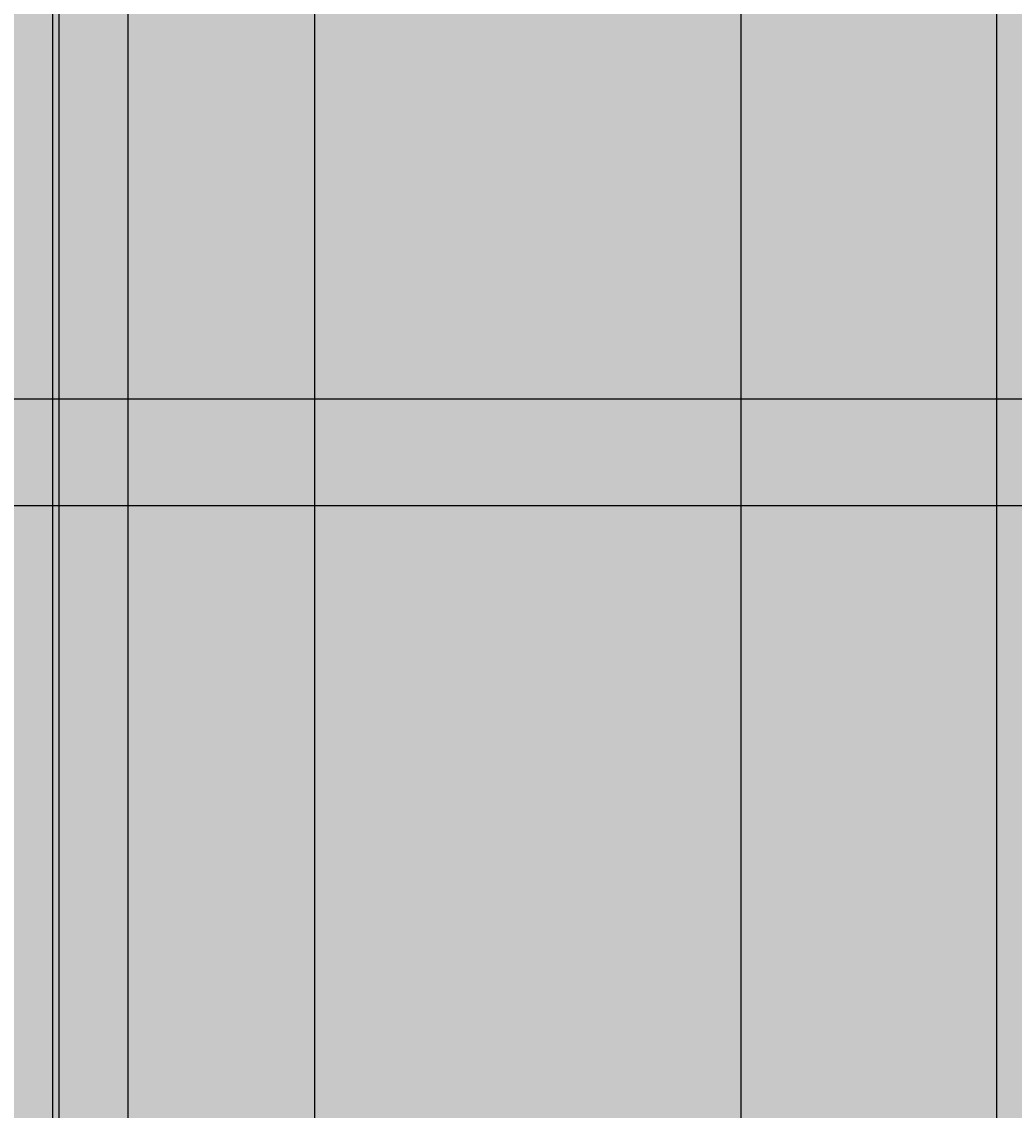
# Model space of a CAD drawing. Units: inches. Extents: x -12 to 334, y -10 to 186.
# Tile 64 of 77: x 216 to 239, y 111 to 137. Entities that reach past the tile are written whole.
import ezdxf

# ---------------------------------------------------------------- set-up
doc = ezdxf.new("R2010")
doc.units = ezdxf.units.IN
doc.header["$MEASUREMENT"] = 0
doc.layers.add('M-DIMS', color=2, linetype='Continuous', lineweight=18)
doc.layers.add('M-EQPM-PATT', color=8, linetype='Continuous', lineweight=18)
doc.styles.get("Standard").update_dxf_attribs({"font": 'arial.ttf'})
doc.dimstyles.get("Standard").update_dxf_attribs({"dimtxt": 0.18, "dimasz": 0.18, "dimexe": 0.18, "dimexo": 0.0625, "dimgap": 0.09, "dimtad": 0, "dimtih": 1, "dimtoh": 1, "dimdec": 4, "dimzin": 0, "dimdsep": 46, "dimtxsty": 'Standard', "dimcen": 0.09, "dimadec": 0, "dimazin": 0, "dimtfac": 1, "dimtdec": 4, "dimtofl": 0, "dimtmove": 0, "dimatfit": 3, "dimfxl": 1, "dimtolj": 1, "dimtzin": 0, "dimarcsym": 0})

# ---------------------------------------------------------------- blocks, each defined once
blk = doc.blocks.new('*D5')
at = {"layer": 'Defpoints', "color": 0, "transparency": 16777216}
for p in [(58.1, 127.708), (58.1, 125.208), (295.976, 125.208)]:
    blk.add_point(p, dxfattribs=at)
at = {"layer": 'M-DIMS', "color": 0, "lineweight": -2, "transparency": 16777216}
for p, q in [((58.163, 127.708), (296.156, 127.708)), ((295.976, 127.528), (295.976, 126.64)), ((295.976, 125.388), (295.976, 126.276)), ((58.163, 125.208), (296.156, 125.208))]:
    blk.add_line(p, q, dxfattribs=at)
at = {"layer": 'M-DIMS', "color": 0, "transparency": 16777216}
for points in [[(295.946, 127.528), (296.006, 127.528), (295.976, 127.708)], [(295.946, 125.388), (296.006, 125.388), (295.976, 125.208)]]:
    blk.add_solid(points, dxfattribs=at)
at = {"layer": 'M-DIMS', "color": 0, "transparency": 16777216, "insert": (295.976, 126.458), "char_height": 0.18, "attachment_point": 5}
blk.add_mtext('\\A1;2.5', dxfattribs=at)
blk = doc.blocks.new('*D27')
at = {"layer": 'Defpoints', "color": 0, "transparency": 16777216}
for p in [(238.576, 169.385), (216.576, 32.854), (238.576, 32.854)]:
    blk.add_point(p, dxfattribs=at)
at = {"layer": 'M-DIMS', "color": 0, "lineweight": -2, "transparency": 16777216}
for p, q in [((216.576, 32.917), (216.576, 169.565)), ((238.576, 32.917), (238.576, 169.565)), ((216.756, 169.385), (227.357, 169.385)), ((238.396, 169.385), (227.796, 169.385))]:
    blk.add_line(p, q, dxfattribs=at)
at = {"layer": 'M-DIMS', "color": 0, "transparency": 16777216}
for points in [[(216.756, 169.415), (216.756, 169.355), (216.576, 169.385)], [(238.396, 169.415), (238.396, 169.355), (238.576, 169.385)]]:
    blk.add_solid(points, dxfattribs=at)
at = {"layer": 'M-DIMS', "color": 0, "transparency": 16777216, "insert": (227.576, 169.385), "char_height": 0.18, "attachment_point": 5}
blk.add_mtext('\\A1;22', dxfattribs=at)
blk = doc.blocks.new('*D28')
at = {"layer": 'Defpoints', "color": 0, "transparency": 16777216}
for p in [(232.576, 169.385), (222.576, 30.854), (232.576, 30.854)]:
    blk.add_point(p, dxfattribs=at)
at = {"layer": 'M-DIMS', "color": 0, "lineweight": -2, "transparency": 16777216}
for p, q in [((222.576, 30.917), (222.576, 169.565)), ((232.576, 30.917), (232.576, 169.565)), ((222.756, 169.385), (227.366, 169.385)), ((232.396, 169.385), (227.786, 169.385))]:
    blk.add_line(p, q, dxfattribs=at)
at = {"layer": 'M-DIMS', "color": 0, "transparency": 16777216}
for points in [[(222.756, 169.415), (222.756, 169.355), (222.576, 169.385)], [(232.396, 169.415), (232.396, 169.355), (232.576, 169.385)]]:
    blk.add_solid(points, dxfattribs=at)
at = {"layer": 'M-DIMS', "color": 0, "transparency": 16777216, "insert": (227.576, 169.385), "char_height": 0.18, "attachment_point": 5}
blk.add_mtext('\\A1;10', dxfattribs=at)
blk = doc.blocks.new('*D34')
at = {"layer": 'Defpoints', "color": 0, "transparency": 16777216}
for p in [(218.192, 169.385), (216.428, 98.108), (218.192, 98.108)]:
    blk.add_point(p, dxfattribs=at)
at = {"layer": 'M-DIMS', "color": 0, "lineweight": -2, "transparency": 16777216}
for p, q in [((216.428, 98.171), (216.428, 169.565)), ((218.192, 98.171), (218.192, 169.565)), ((216.608, 169.385), (216.995, 169.385)), ((218.012, 169.385), (217.625, 169.385))]:
    blk.add_line(p, q, dxfattribs=at)
at = {"layer": 'M-DIMS', "color": 0, "transparency": 16777216}
for points in [[(216.608, 169.415), (216.608, 169.355), (216.428, 169.385)], [(218.012, 169.415), (218.012, 169.355), (218.192, 169.385)]]:
    blk.add_solid(points, dxfattribs=at)
at = {"layer": 'M-DIMS', "color": 0, "transparency": 16777216, "insert": (217.31, 169.385), "char_height": 0.18, "attachment_point": 5}
blk.add_mtext('\\A1;1.76', dxfattribs=at)
blk = doc.blocks.new('*D37')
at = {"layer": 'Defpoints', "color": 0, "transparency": 16777216}
for p in [(245.935, 169.385), (232.576, 46.854), (245.935, 46.854)]:
    blk.add_point(p, dxfattribs=at)
at = {"layer": 'M-DIMS', "color": 0, "lineweight": -2, "transparency": 16777216}
for p, q in [((232.576, 46.917), (232.576, 169.565)), ((245.935, 46.917), (245.935, 169.565)), ((232.756, 169.385), (238.871, 169.385)), ((245.755, 169.385), (239.641, 169.385))]:
    blk.add_line(p, q, dxfattribs=at)
at = {"layer": 'M-DIMS', "color": 0, "transparency": 16777216}
for points in [[(232.756, 169.415), (232.756, 169.355), (232.576, 169.385)], [(245.755, 169.415), (245.755, 169.355), (245.935, 169.385)]]:
    blk.add_solid(points, dxfattribs=at)
at = {"layer": 'M-DIMS', "color": 0, "transparency": 16777216, "insert": (239.256, 169.385), "char_height": 0.18, "attachment_point": 5}
blk.add_mtext('\\A1;13.36', dxfattribs=at)
blk = doc.blocks.new('*D40')
at = {"layer": 'Defpoints', "color": 0, "transparency": 16777216}
for p in [(278.229, 116.208), (187.394, 91.899)]:
    blk.add_point(p, dxfattribs=at)
at = {"layer": 'M-DIMS', "color": 0, "lineweight": -2, "transparency": 16777216}
for p, q in [((332.73, 130.793), (278.403, 116.254)), ((187.394, 91.809), (187.394, 91.989)), ((187.304, 91.899), (187.484, 91.899))]:
    blk.add_line(p, q, dxfattribs=at)
at = {"layer": 'M-DIMS', "color": 0, "transparency": 16777216}
blk.add_solid([(278.395, 116.283), (278.411, 116.225), (278.229, 116.208)], dxfattribs=at)
at = {"layer": 'M-DIMS', "color": 0, "transparency": 16777216, "insert": (333.21, 130.793), "char_height": 0.18, "attachment_point": 5}
blk.add_mtext('\\A1;R94.03', dxfattribs=at)

msp = doc.modelspace()

# ---------------------------------------------------------------- hatches: boundary and pattern name
at = {"layer": 'M-EQPM-PATT', "transparency": 33554556}
h = msp.add_hatch(color=256, dxfattribs=at)
h.set_gradient(color1=(248, 206, 179), color2=(248, 206, 179), tint=1)
h.paths.add_polyline_path([(179.7818, 136.8871), (126.9567, 136.8871), (106.1771, 100.8958), (171.5458, 100.8958)])
h.paths.add_polyline_path([(268.3808, 136.9435), (214.0166, 136.9435), (214.0166, 154.8345), (196.3421, 154.8345), (196.3421, 136.8871), (179.7818, 136.8871), (171.5458, 100.8958), (231.7758, 100.8958, -0.4142136), (251.9801, 80.6915), (279.7263, 80.6915, 0.1631825)])

# ---------------------------------------------------------------- dimensions: what is measured, and where the dimension line sits
at = {"layer": 'M-DIMS'}
for base, p1, p2, override, picture, middle in [((218.1922, 169.3845), (216.4278, 98.1081), (218.1922, 98.1081), {"dimdec": 2, "dimlfac": 1, "dimrnd": 0, "dimzin": 0, "dimdsep": 46, "dimlunit": 2}, '*D34', (217.31, 169.3845)), ((238.5761, 169.3845), (216.5761, 32.8541), (238.5761, 32.8541), {"dimdec": 0, "dimlfac": 1, "dimrnd": 0, "dimzin": 0, "dimdsep": 46, "dimlunit": 2}, '*D27', (227.5761, 169.3845)), ((232.5761, 169.3845), (222.5761, 30.8541), (232.5761, 30.8541), {"dimdec": 0, "dimlfac": 1, "dimrnd": 0, "dimzin": 0, "dimdsep": 46, "dimlunit": 2}, '*D28', (227.5761, 169.3845)), ((245.9354, 169.3845), (232.5761, 46.8541), (245.9354, 46.8541), {"dimdec": 2, "dimlfac": 1, "dimrnd": 0, "dimzin": 0, "dimdsep": 46, "dimlunit": 2}, '*D37', (239.2558, 169.3845))]:
    dim = msp.add_linear_dim(base=base, p1=p1, p2=p2, dimstyle='Standard', override=override, dxfattribs=at)
    dim.commit()
    dim.dimension.update_dxf_attribs({"geometry": picture, "text_midpoint": middle})
dim = msp.add_radius_dim(center=(187.3936, 91.8988), mpoint=(278.2291, 116.2078), dimstyle='Standard', override={"dimdec": 2, "dimlfac": 1, "dimrnd": 0, "dimzin": 0, "dimdsep": 46, "dimlunit": 2}, dxfattribs=at)
dim.commit()
dim.dimension.update_dxf_attribs({"geometry": '*D40', "text_midpoint": (332.7304, 130.7932), "dimtype": 164})
dim = msp.add_linear_dim(base=(295.9756, 125.2078), p1=(58.1002, 127.7078), p2=(58.1002, 125.2078), angle=90, dimstyle='Standard', override={"dimdec": 1, "dimlfac": 1, "dimrnd": 0, "dimzin": 0, "dimdsep": 46, "dimlunit": 2}, dxfattribs=at)
dim.commit()
dim.dimension.update_dxf_attribs({"geometry": '*D5', "text_midpoint": (295.9756, 126.4578)})

doc.saveas('drawing.dxf')
